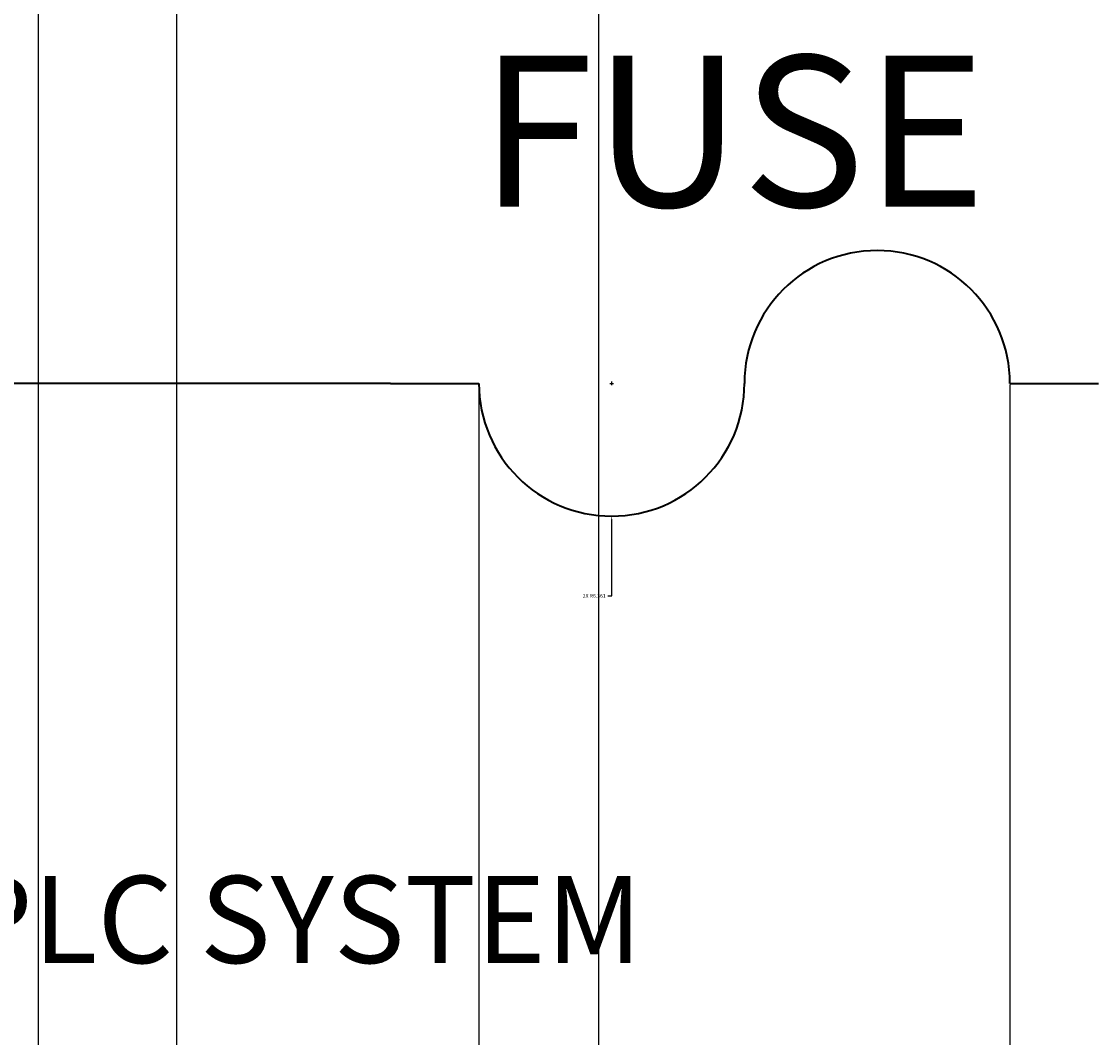
# Model space of a CAD drawing. Units: inches. Extents: x 738 to 1068, y 378 to 757.
# Tile 37 of 41: x 809 to 860, y 655 to 704. Entities that reach past the tile are written whole.
import ezdxf

# ---------------------------------------------------------------- set-up
doc = ezdxf.new("R2010")
doc.units = ezdxf.units.IN
doc.header["$MEASUREMENT"] = 0
for name, color, linetype, lineweight in [('A-ANNO-DIMS', 2, 'Continuous', 18), ('E-ANNO-TEXT', 7, 'Continuous', 18), ('E-POWR-EQPM', 4, 'Continuous', 35), ('E-POWR-FEED', 7, 'Continuous', 35)]:
    doc.layers.add(name, color=color, linetype=linetype, lineweight=lineweight)
doc.styles.get("Standard").update_dxf_attribs({"font": 'arial.ttf'})
doc.dimstyles.get("Standard").update_dxf_attribs({"dimtxt": 0.18, "dimasz": 0.18, "dimexe": 0.18, "dimexo": 0.0625, "dimgap": 0.09, "dimtad": 0, "dimtih": 1, "dimtoh": 1, "dimdec": 4, "dimzin": 0, "dimdsep": 46, "dimtxsty": 'Standard', "dimcen": 0.09, "dimadec": 0, "dimazin": 0, "dimtfac": 1, "dimtdec": 4, "dimtofl": 0, "dimtmove": 0, "dimatfit": 3, "dimfxl": 1, "dimtolj": 1, "dimtzin": 0, "dimarcsym": 0})

# ---------------------------------------------------------------- blocks, each defined once
blk = doc.blocks.new('Fuse')
for p, q in [((0, 0), (0.05, 0)), ((0.35, 0), (0.4, 0))]:
    blk.add_line(p, q)
for centre, start, end in [((0.275, 0), 0, 180), ((0.125, 0), 180, 0)]:
    blk.add_arc(centre, 0.075, start, end)
blk = doc.blocks.new('*D26')
at = {"layer": 'A-ANNO-DIMS', "color": 0, "lineweight": -2, "transparency": 16777216}
for p, q in [((816.008, 647.048), (816.008, 756.505)), ((867.596, 647.048), (867.596, 756.505)), ((816.188, 756.325), (841.408, 756.325)), ((867.416, 756.325), (842.196, 756.325))]:
    blk.add_line(p, q, dxfattribs=at)
at = {"layer": 'A-ANNO-DIMS', "color": 0, "transparency": 16777216}
for points in [[(816.188, 756.355), (816.188, 756.295), (816.008, 756.325)], [(867.416, 756.355), (867.416, 756.295), (867.596, 756.325)]]:
    blk.add_solid(points, dxfattribs=at)
at = {"layer": 'Defpoints', "color": 0, "transparency": 16777216}
for p in [(867.596, 756.325), (816.008, 646.985), (867.596, 646.985)]:
    blk.add_point(p, dxfattribs=at)
at = {"layer": 'A-ANNO-DIMS', "color": 0, "transparency": 16777216, "insert": (841.802, 756.325), "char_height": 0.18, "attachment_point": 5}
blk.add_mtext('\\A1;51.59', dxfattribs=at)
blk = doc.blocks.new('*D32')
at = {"layer": 'A-ANNO-DIMS', "color": 0, "lineweight": -2, "transparency": 16777216}
for p, q in [((809.38, 461.454), (809.38, 756.505)), ((836.232, 461.277), (836.232, 756.505)), ((809.56, 756.325), (822.41, 756.325)), ((836.052, 756.325), (823.202, 756.325))]:
    blk.add_line(p, q, dxfattribs=at)
at = {"layer": 'A-ANNO-DIMS', "color": 0, "transparency": 16777216}
for points in [[(809.56, 756.355), (809.56, 756.295), (809.38, 756.325)], [(836.052, 756.355), (836.052, 756.295), (836.232, 756.325)]]:
    blk.add_solid(points, dxfattribs=at)
at = {"layer": 'Defpoints', "color": 0, "transparency": 16777216}
for p in [(836.232, 756.325), (809.38, 461.392), (836.232, 461.214)]:
    blk.add_point(p, dxfattribs=at)
at = {"layer": 'A-ANNO-DIMS', "color": 0, "transparency": 16777216, "insert": (822.806, 756.325), "char_height": 0.18, "attachment_point": 5}
blk.add_mtext('\\A1;26.85', dxfattribs=at)
blk = doc.blocks.new('*D34')
at = {"layer": 'A-ANNO-DIMS', "color": 0, "lineweight": -2, "transparency": 16777216}
for p, q in [((781.49, 686.266), (781.49, 378.239)), ((830.489, 686.266), (830.489, 378.239)), ((781.67, 378.419), (805.767, 378.419)), ((830.309, 378.419), (806.212, 378.419))]:
    blk.add_line(p, q, dxfattribs=at)
at = {"layer": 'A-ANNO-DIMS', "color": 0, "transparency": 16777216}
for points in [[(781.67, 378.449), (781.67, 378.389), (781.49, 378.419)], [(830.309, 378.449), (830.309, 378.389), (830.489, 378.419)]]:
    blk.add_solid(points, dxfattribs=at)
at = {"layer": 'Defpoints', "color": 0, "transparency": 16777216}
for p in [(781.49, 686.329), (830.489, 686.329), (830.489, 378.419)]:
    blk.add_point(p, dxfattribs=at)
at = {"layer": 'A-ANNO-DIMS', "color": 0, "transparency": 16777216, "insert": (805.99, 378.419), "char_height": 0.18, "attachment_point": 5}
blk.add_mtext('\\A1;49', dxfattribs=at)
blk = doc.blocks.new('*D35')
at = {"layer": 'A-ANNO-DIMS', "color": 0, "lineweight": -2, "transparency": 16777216}
for p, q in [((855.932, 686.266), (855.932, 378.239)), ((901.429, 686.267), (901.429, 378.239)), ((856.112, 378.419), (878.352, 378.419)), ((901.249, 378.419), (879.009, 378.419))]:
    blk.add_line(p, q, dxfattribs=at)
at = {"layer": 'A-ANNO-DIMS', "color": 0, "transparency": 16777216}
for points in [[(856.112, 378.449), (856.112, 378.389), (855.932, 378.419)], [(901.249, 378.449), (901.249, 378.389), (901.429, 378.419)]]:
    blk.add_solid(points, dxfattribs=at)
at = {"layer": 'Defpoints', "color": 0, "transparency": 16777216}
for p in [(855.932, 686.329), (901.429, 686.329), (901.429, 378.419)]:
    blk.add_point(p, dxfattribs=at)
at = {"layer": 'A-ANNO-DIMS', "color": 0, "transparency": 16777216, "insert": (878.68, 378.419), "char_height": 0.18, "attachment_point": 5}
blk.add_mtext('\\A1;45.5', dxfattribs=at)
blk = doc.blocks.new('*D41')
at = {"layer": 'A-ANNO-DIMS', "color": 0, "lineweight": -2, "transparency": 16777216}
for p, q in [((836.76, 686.329), (836.94, 686.329)), ((836.85, 686.239), (836.85, 686.419)), ((836.85, 676.152), (836.85, 679.788)), ((836.67, 676.152), (836.85, 676.152))]:
    blk.add_line(p, q, dxfattribs=at)
at = {"layer": 'A-ANNO-DIMS', "color": 0, "transparency": 16777216}
blk.add_solid([(836.82, 679.788), (836.88, 679.788), (836.85, 679.968)], dxfattribs=at)
at = {"layer": 'Defpoints', "color": 0, "transparency": 16777216}
for p in [(836.85, 686.329), (836.85, 679.968)]:
    blk.add_point(p, dxfattribs=at)
at = {"layer": 'A-ANNO-DIMS', "color": 0, "transparency": 16777216, "insert": (836.013, 676.152), "char_height": 0.18, "attachment_point": 5}
blk.add_mtext('\\A1;2X R6.361', dxfattribs=at)

msp = doc.modelspace()

# ---------------------------------------------------------------- linework, layer by layer
at = {"layer": 'E-POWR-FEED'}
msp.add_line((826.2488, 686.329), (781.4897, 686.329), dxfattribs=at)

# ---------------------------------------------------------------- block references
at = {"layer": 'E-POWR-EQPM', "xscale": 84.80997268620614, "yscale": 84.80997268620614, "zscale": 84.80997268620614}
msp.add_blockref('Fuse', (826.2488, 686.329), dxfattribs=at)

# ---------------------------------------------------------------- texts
at = {"layer": 'E-ANNO-TEXT'}
for s, height, p in [('FUSE', 7.24182, (830.5089, 694.786)), ('STOP PLC SYSTEM', 4.175074, (789.5941, 658.5662))]:
    msp.add_text(s, height=height, dxfattribs=at).set_placement(p)

# ---------------------------------------------------------------- dimensions: what is measured, and where the dimension line sits
at = {"layer": 'A-ANNO-DIMS'}
for base, p1, p2, override, picture, middle in [((836.2324, 756.3251), (809.3803, 461.3919), (836.2324, 461.214), {"dimdec": 2, "dimlfac": 1, "dimrnd": 0, "dimzin": 0, "dimdsep": 46, "dimlunit": 2}, '*D32', (822.8064, 756.3251)), ((867.5964, 756.3251), (816.0076, 646.9853), (867.5964, 646.9853), {"dimdec": 2, "dimlfac": 1, "dimrnd": 0, "dimzin": 0, "dimdsep": 46, "dimlunit": 2}, '*D26', (841.802, 756.3251)), ((830.4893, 378.4191), (781.4897, 686.329), (830.4893, 686.329), {"dimdec": 0, "dimlfac": 1, "dimrnd": 0, "dimzin": 0, "dimdsep": 46, "dimlunit": 2}, '*D34', (805.9895, 378.4191)), ((901.4286, 378.4191), (855.9323, 686.329), (901.4286, 686.3292), {"dimdec": 1, "dimlfac": 1, "dimrnd": 0, "dimzin": 0, "dimdsep": 46, "dimlunit": 2}, '*D35', (878.6804, 378.4191))]:
    dim = msp.add_linear_dim(base=base, p1=p1, p2=p2, dimstyle='Standard', override=override, dxfattribs=at)
    dim.commit()
    dim.dimension.update_dxf_attribs({"geometry": picture, "text_midpoint": middle})
dim = msp.add_radius_dim(center=(836.8501, 686.329), mpoint=(836.85, 679.9682), text='2X <>', dimstyle='Standard', override={"dimdec": 3, "dimlfac": 1, "dimrnd": 0, "dimzin": 0, "dimdsep": 46, "dimlunit": 2}, dxfattribs=at)
dim.commit()
dim.dimension.update_dxf_attribs({"geometry": '*D41', "text_midpoint": (836.0126, 676.1518), "dimtype": 164})

doc.saveas('drawing.dxf')
